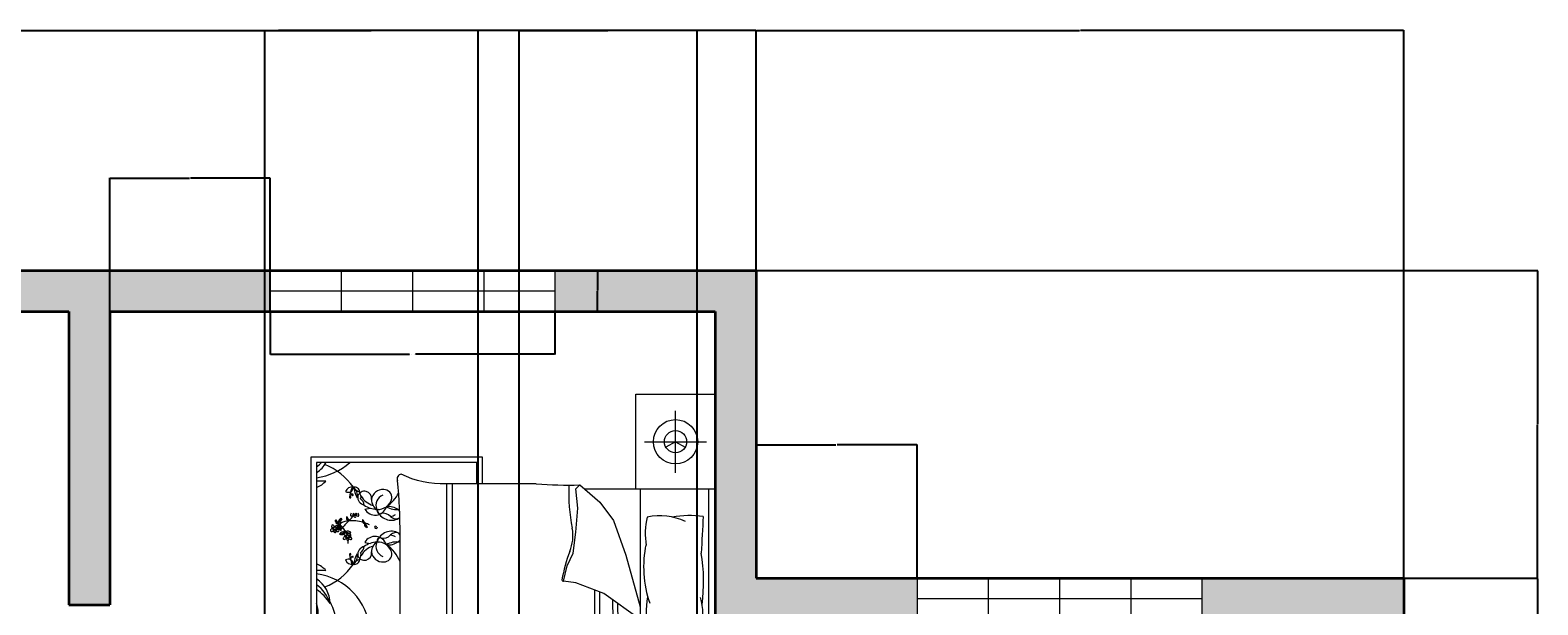
# Model space of a CAD drawing. Units: centimetres. Extents: x 2178 to 3635, y 1064 to 2635.
# Tile 9 of 9: x 2788 to 3635, y 2312 to 2635. Entities that reach past the tile are written whole.
import ezdxf

# ---------------------------------------------------------------- set-up
doc = ezdxf.new("R2010")
doc.units = ezdxf.units.CM
for name, color, linetype, lineweight in [('A-ANNO-DIMS', 2, 'Continuous', 18), ('A-FURN', 42, 'Continuous', 18), ('A-GLAZ', 4, 'Continuous', 18), ('A-WALL', 7, 'Continuous', 35)]:
    doc.layers.add(name, color=color, linetype=linetype, lineweight=lineweight)
doc.layers.add('A-WALL-PATT', color=18, linetype='Continuous', lineweight=13, true_color=0x000000)
doc.styles.get("Standard").update_dxf_attribs({"font": 'arial.ttf'})
doc.dimstyles.get("Standard").update_dxf_attribs({"dimtxt": 0.18, "dimasz": 0.18, "dimexe": 0.18, "dimexo": 0.0625, "dimgap": 0.09, "dimtad": 0, "dimtih": 1, "dimtoh": 1, "dimdec": 4, "dimzin": 0, "dimdsep": 46, "dimtxsty": 'Standard', "dimcen": 0.09, "dimadec": 0, "dimazin": 0, "dimtfac": 1, "dimtdec": 4, "dimtofl": 0, "dimtmove": 0, "dimatfit": 3, "dimfxl": 1, "dimtolj": 1, "dimtzin": 0, "dimarcsym": 0})

# ---------------------------------------------------------------- blocks, each defined once
blk = doc.blocks.new('bed')
for p, q in [((2798.77, 2937.13), (3098.77, 2937.13)), ((2858.77, 2937.13), (2858.77, 2854.79)), ((3038.77, 2933.28), (2858.77, 2933.28)), ((2828.77, 2892.53), (2828.77, 2931.73)), ((3068.77, 2892.53), (3068.77, 2931.73)), ((2848.37, 2912.13), (2809.17, 2912.13)), ((3049.17, 2912.13), (3088.37, 2912.13)), ((2858.77, 2889.72), (3038.77, 2889.72)), ((2900.44, 2880.8), (2933.16, 2889.72)), ((2941.19, 2889.72), (2924.75, 2866.84)), ((2878.57, 2872.91), (2900.44, 2880.8)), ((3037.97, 2877.26), (2931.16, 2875.76)), ((2867.02, 2864.41), (2878.57, 2872.91)), ((2924.75, 2866.84), (2918.06, 2849.23)), ((3037.85, 2874.18), (2928.92, 2872.64)), ((2856.09, 2851.66), (2867.02, 2864.41)), ((3037.71, 2861.65), (2922.6, 2861.18)), ((3037.69, 2864.73), (2923.78, 2864.28)), ((2858.52, 2849.23), (2856.09, 2851.66)), ((2870.67, 2850.44), (2858.52, 2849.23)), ((2885.86, 2849.23), (2870.67, 2850.44)), ((2899.23, 2847.41), (2885.86, 2849.23)), ((2907.13, 2843.76), (2899.23, 2847.41)), ((2918.06, 2849.23), (2916.85, 2841.33)), ((2916.85, 2841.33), (2907.13, 2843.76)), ((2838.37, 2790.07), (2855.34, 2790.07)), ((2838.37, 2682), (2838.37, 2790.07)), ((3040.44, 2790.07), (3057.08, 2790.07)), ((3057.08, 2790.07), (3057.08, 2682)), ((2855.33, 2786.59), (2841.85, 2786.59)), ((2841.85, 2786.59), (2841.85, 2685.48)), ((3053.6, 2786.59), (3040.38, 2786.59)), ((3053.6, 2685.48), (3053.6, 2786.59)), ((3040.13, 2771.36), (2855.32, 2771.36)), ((3040.42, 2767.62), (2855.31, 2767.62)), ((3009.67, 2738.15), (2887.87, 2738.15)), ((2871.41, 2715.89), (2870.75, 2719.28)), ((2892.38, 2715.89), (2893.04, 2719.28)), ((3003.07, 2715.89), (3002.41, 2719.28)), ((3024.04, 2715.89), (3024.7, 2719.28)), ((2841.85, 2685.48), (3053.6, 2685.48)), ((3057.08, 2682), (2838.37, 2682))]:
    blk.add_line(p, q)
for points in [[(2858.77, 2887.13), (2798.77, 2887.13), (2798.77, 2937.13)], [(3038.77, 2937.13), (3038.77, 2887.13), (3098.77, 2887.13), (3098.77, 2937.13)], [(2828.77, 2912.13), (2832.27, 2918.19)], [(3068.77, 2912.13), (3065.27, 2918.19)], [(2828.77, 2912.13), (2832.27, 2906.07)], [(3068.77, 2912.13), (3065.27, 2906.07)]]:
    blk.add_lwpolyline(points)
for points in [[(2876, 2929.65, 0.074897), (2876.37, 2910.06, -0.472817)], [(2947.37, 2908.96, 0.14099), (2947.97, 2928.95, 0.235245)], [(2960.18, 2908.96, -0.14099), (2959.58, 2928.95, -0.235245)], [(3021.54, 2929.65, -0.074897), (3021.18, 2910.06, 0.472817)], [(2855.46, 2824.19, 0.001242), (2855.31, 2767.26, -0.127202), (2849.3, 2738.9)], [(3040.05, 2773.72, 0.056112), (3042.23, 2757.21, 0.095341), (3046.45, 2741.32)]]:
    blk.add_lwpolyline(points, format="xyb")
for centre, radius in [((2828.77, 2912.13), 14), ((3068.77, 2912.13), 14), ((2828.77, 2912.13), 7), ((3068.77, 2912.13), 7), ((2888.74, 2705.02), 0.764), ((3006.71, 2705.02), 0.764), ((2883.74, 2696.97), 0.764), ((3011.71, 2696.97), 0.764)]:
    blk.add_circle(centre, radius)
for centre, radius, start, end in [((3041.36, 5784.66), 2859.79, 266.68521, 267.14978), ((2917.11, 2821.09), 108.8, 82.21958, 99.49698), ((2940.09, 2876.08), 53.46, 81.52493, 103.95996), ((2963.69, 2914.69), 14.84, 63.34374, 106.10256), ((2985.93, 2877.16), 52.74, 76.34271, 101.1841), ((2856.18, 5784.66), 2859.79, 272.85022, 273.31479), ((2914.22, 2902.19), 38.67, 155.1316, 191.75834), ((2983.32, 2902.19), 38.67, 348.24166, 24.8684), ((2912, 2898.93), 36.76, 354.01289, 15.82928), ((2995.54, 2898.93), 36.76, 164.17072, 185.98711), ((2907.87, 2961.74), 69.73, 258.03974, 289.26152), ((2936.1, 2946.52), 52.9, 259.86169, 283.62376), ((2965.7, 2909.52), 15.9, 245.01826, 288.54073), ((2993.49, 2930.2), 38.19, 243.87611, 286.17464), ((2886.7, 2933.16), 40.2, 255.10393, 281.03689), ((3010.84, 2933.16), 40.2, 258.96311, 284.89607), ((3576.57, 2853.06), 539.05, 176.09997, 180.92818), ((2581.02, 2844.2), 275.17, 355.82941, 1.55305), ((2888.28, 2822.94), 24.42, 66.26158, 101.3392), ((2861.22, 2957.89), 113.22, 267.45188, 281.3392), ((2937.68, 2954.7), 116.34, 250.11942, 259.33829), ((2916.17, 2841.09), 0.724, 268.86235, 19.75363), ((3740.68, 2833.46), 703.17, 179.11454, 184.87351), ((2852.06, 2739.09), 2.77, 183.97998, 297.34124), ((2884.29, 2425.86), 312.3, 89.34325, 95.68869), ((2864.12, 2727.92), 5.07, 84.48557, 181.05378), ((2850.89, 2717.02), 22.71, 33.66712, 63.29966), ((2862.56, 2724.18), 9.02, 355.29334, 76.921), ((2881.32, 2730.53), 11.57, 145.78505, 184.73037), ((2859.22, 2735.93), 12.43, 328.82178, 9.15542), ((2874.61, 2734.83), 3.61, 120.0293, 142.32497), ((2868.85, 2732.7), 9.56, 289.28218, 29.1751), ((2867.4, 2730.97), 8.62, 7.43599, 29.91487), ((2873.09, 2735.54), 4.49, 311.56531, 23.83541), ((2874.61, 2734.83), 3.61, 44.45169, 63.55801), ((2894.94, 2732.7), 9.56, 150.8249, 250.71782), ((2890.7, 2735.54), 4.49, 156.16459, 228.43469), ((2889.17, 2734.83), 3.61, 113.22901, 135.54831), ((2896.38, 2730.97), 8.62, 150.08513, 172.56401), ((2889.17, 2734.83), 3.61, 37.67503, 66.71436), ((2882.46, 2730.53), 11.57, 355.26963, 34.21495), ((2904.56, 2735.93), 12.43, 169.71335, 211.17822), ((2901.22, 2724.18), 9.02, 103.079, 184.70666), ((2912.89, 2717.02), 22.71, 111.49413, 146.33288), ((2899.66, 2727.92), 5.07, 358.94622, 95.51443), ((2995.79, 2727.92), 5.07, 84.48557, 181.05378), ((2982.56, 2717.02), 22.71, 33.66712, 68.50587), ((2994.23, 2724.18), 9.02, 355.29334, 76.921), ((3012.99, 2730.53), 11.57, 145.78505, 184.73037), ((2990.89, 2735.93), 12.43, 328.82178, 10.28665), ((3006.28, 2734.83), 3.61, 113.28564, 142.32497), ((3000.51, 2732.7), 9.56, 289.28218, 29.1751), ((2999.07, 2730.97), 8.62, 7.43599, 29.91487), ((3006.28, 2734.83), 3.61, 44.45169, 66.71436), ((3004.75, 2735.54), 4.49, 311.56531, 23.83541), ((3018.86, 2446.37), 291.92, 85.24024, 91.80351), ((3026.6, 2732.7), 9.56, 150.8249, 250.71782), ((3022.36, 2735.54), 4.49, 156.16459, 228.43469), ((3020.84, 2734.83), 3.61, 106.63434, 135.54831), ((3028.05, 2730.97), 8.62, 150.08513, 172.56401), ((3020.84, 2734.83), 3.61, 37.67503, 72.58143), ((3014.13, 2730.53), 11.57, 355.26963, 34.21495), ((3036.23, 2735.93), 12.43, 169.24899, 211.17822), ((3032.89, 2724.18), 9.02, 103.079, 184.70666), ((3044.56, 2717.02), 22.71, 113.64533, 146.33288), ((3031.33, 2727.92), 5.07, 358.94622, 95.51443), ((3044.17, 2739.79), 2.73, 246.52186, 33.82642), ((2866.2, 2727.2), 7.17, 174.94485, 262.88575), ((2869.01, 2729.92), 6.96, 201.58187, 291.42215), ((2864.95, 2728.79), 8.71, 272.3591, 324.04014), ((2855.49, 2724.42), 16.1, 326.28828, 356.5076), ((2867.69, 2722.36), 7.46, 299.90854, 73.1337), ((2881.32, 2730.53), 11.57, 212.70113, 216.34448), ((2872.41, 2725.49), 1.86, 257.30406, 15.14713), ((2880.15, 2727.58), 6.15, 131.56531, 195.14713), ((2882.69, 2723.02), 0.94, 280.43845, 100.41356), ((2883.64, 2727.58), 6.15, 344.85287, 48.43469), ((2896.09, 2722.36), 7.46, 106.8663, 240.09146), ((2891.37, 2725.49), 1.86, 164.85287, 282.69594), ((2882.46, 2730.53), 11.57, 323.65552, 327.29887), ((2898.83, 2728.79), 8.71, 215.95986, 267.6409), ((2894.77, 2729.92), 6.96, 248.57785, 338.41813), ((2908.3, 2724.42), 16.1, 183.4924, 213.71172), ((2897.59, 2727.2), 7.17, 277.11425, 5.05515), ((2997.86, 2727.2), 7.17, 174.94485, 262.88575), ((3000.68, 2729.92), 6.96, 201.58187, 291.42215), ((2996.62, 2728.79), 8.71, 272.3591, 324.04014), ((2987.15, 2724.42), 16.1, 326.28828, 356.5076), ((2999.36, 2722.36), 7.46, 299.90854, 73.1337), ((3012.99, 2730.53), 11.57, 212.70113, 216.34448), ((3004.08, 2725.49), 1.86, 257.30406, 15.14713), ((3011.81, 2727.58), 6.15, 131.56531, 195.14713), ((3012.76, 2723.02), 0.94, 79.58644, 259.56155), ((3015.3, 2727.58), 6.15, 344.85287, 48.43469), ((3027.76, 2722.36), 7.46, 106.8663, 240.09146), ((3023.04, 2725.49), 1.86, 164.85287, 282.69594), ((3014.13, 2730.53), 11.57, 323.65552, 327.29887), ((3030.5, 2728.79), 8.71, 215.95986, 267.6409), ((3026.44, 2729.92), 6.96, 248.57785, 338.41813), ((3039.96, 2724.42), 16.1, 183.4924, 213.71172), ((3029.25, 2727.2), 7.17, 277.11425, 5.05515), ((2864.55, 2715.65), 4.5, 80.26398, 250.86884), ((2855.62, 2725.56), 14.16, 301.26137, 341.7045), ((2863.47, 2717), 5.62, 265.96902, 344.3045), ((2869.52, 2709.53), 5.99, 96.1662, 141.58255), ((2879.44, 2713.73), 1.58, 101.32561, 154.46214), ((2877.17, 2719.07), 4.74, 280.25878, 300.65599), ((2878.27, 2722.86), 8.46, 268.32639, 277.13024), ((2903.55, 2707.57), 24.85, 163.58418, 183.82768), ((2876.15, 2719.06), 4.82, 308.21012, 316.30712), ((2879.11, 2715.89), 1.44, 278.34322, 4.28685), ((2878.31, 2717.16), 2.51, 300.65599, 332.63414), ((2880.2, 2715.5), 0.611, 55.76575, 157.44165), ((2903.55, 2707.57), 24.85, 153.0032, 159.89408), ((2881.15, 2716.07), 0.611, 84.37838, 186.05427), ((2880.58, 2718.52), 2.51, 269.18588, 301.16403), ((2881.32, 2717.22), 1.44, 237.53317, 323.47681), ((2879.92, 2721.32), 4.82, 285.51291, 293.60991), ((2883.07, 2715.9), 1.58, 87.35788, 140.49441), ((2879.43, 2720.42), 4.74, 301.16403, 321.56124), ((2882.75, 2722.67), 0.578, 102.70507, 280.43845), ((2875.57, 2721.25), 8.46, 324.68979, 333.49364), ((2908.16, 2725.56), 14.16, 198.2955, 238.73863), ((2894.26, 2709.53), 5.99, 38.41745, 83.8338), ((2900.32, 2717), 5.62, 195.6955, 274.03098), ((2899.24, 2715.65), 4.5, 289.13116, 99.73602), ((2951.1, 2680.2), 39.18, 94.46233, 172.25504), ((2951.27, 2716.33), 4.34, 137.78732, 219.11446), ((2946.34, 2716.47), 3.27, 298.5391, 58.36268), ((2951.26, 2719.13), 3.2, 177.75849, 283.85198), ((2951.17, 2718.35), 3.25, 63.02737, 163.80375), ((2947.89, 2725.94), 6.69, 271.45846, 315.37266), ((2950.61, 2713.61), 6.19, 45.54113, 114.31008), ((2956.25, 2745.4), 27.41, 252.59304, 267.25817), ((2957.43, 2722.47), 9.91, 198.91595, 238.01098), ((2954.84, 2713.61), 6.19, 65.68992, 134.45887), ((2949.2, 2745.4), 27.41, 272.74183, 287.40696), ((2951.92, 2716.43), 0.424, 283.85198, 219.92454), ((2952.44, 2714.47), 0.487, 238.01098, 71.55918), ((2952.52, 2714.71), 0.236, 71.55918, 188.01668), ((2953.01, 2714.47), 0.487, 108.44082, 301.98902), ((2954.28, 2718.35), 3.25, 16.19625, 116.97263), ((2957.56, 2725.94), 6.69, 224.62734, 268.54154), ((2952.93, 2714.71), 0.236, 351.98332, 108.44082), ((2953.49, 2716.59), 0.255, 320.19092, 256.02088), ((2948.02, 2722.47), 9.91, 301.98902, 341.08405), ((2954.19, 2719.13), 3.2, 256.14802, 2.24151), ((2959.11, 2716.47), 3.27, 121.63732, 241.4609), ((2954.18, 2716.33), 4.34, 320.88554, 42.21268), ((2953.08, 2689.24), 30.32, 352.86355, 81.81966), ((2996.21, 2715.65), 4.5, 80.26398, 250.86884), ((2987.29, 2725.56), 14.16, 301.26137, 341.7045), ((2995.13, 2717), 5.62, 265.96902, 344.3045), ((3001.19, 2709.53), 5.99, 96.1662, 141.58255), ((3012.38, 2715.9), 1.58, 39.50559, 92.64212), ((3016.02, 2720.42), 4.74, 218.43876, 238.83597), ((3019.88, 2721.25), 8.46, 206.50636, 215.31021), ((3012.7, 2722.67), 0.578, 259.56155, 77.29493), ((3014.13, 2717.22), 1.44, 216.52319, 302.46683), ((3014.87, 2718.52), 2.51, 238.83597, 270.81412), ((3015.53, 2721.32), 4.82, 246.39009, 254.48709), ((2991.9, 2707.57), 24.85, 20.10592, 26.9968), ((3014.3, 2716.07), 0.611, 353.94573, 95.62162), ((3016.34, 2715.89), 1.44, 175.71315, 261.65678), ((3015.25, 2715.5), 0.611, 22.55835, 124.23425), ((3017.14, 2717.16), 2.51, 207.36586, 239.34401), ((2991.9, 2707.57), 24.85, 356.17232, 16.41582), ((3019.3, 2719.06), 4.82, 223.69288, 231.78988), ((3018.28, 2719.07), 4.74, 239.34401, 259.74122), ((3017.18, 2722.86), 8.46, 262.86976, 271.67361), ((3016.01, 2713.73), 1.58, 25.53786, 78.67439), ((3039.83, 2725.56), 14.16, 198.2955, 238.73863), ((3031.98, 2717), 5.62, 195.6955, 274.03098), ((3025.93, 2709.53), 5.99, 38.41745, 83.8338), ((3030.9, 2715.65), 4.5, 289.13116, 99.73602), ((2812.68, 2680.2), 39.18, 7.74496, 41.8856), ((2879.7, 2676.32), 39.18, 124.38655, 158.59079), ((2860.73, 2709.42), 3.25, 92.95159, 193.72796), ((2861.82, 2707.73), 4.34, 167.71153, 249.03868), ((2854.09, 2714.37), 6.69, 301.38267, 345.29688), ((2862.6, 2705.03), 6.19, 75.46535, 144.23429), ((2851.64, 2735.41), 27.41, 282.51726, 297.18239), ((2857.48, 2705.38), 3.27, 328.46331, 88.28689), ((2864.1, 2716.11), 9.91, 228.84017, 267.9352), ((2860.42, 2710.14), 3.2, 207.6827, 313.77619), ((2863.62, 2710.77), 2.76, 63.97555, 143.26805), ((2862.34, 2708.13), 0.424, 313.77619, 249.71835), ((2863.71, 2706.94), 0.236, 101.4834, 217.94089), ((2863.76, 2706.7), 0.487, 267.9352, 101.4834), ((2874.99, 2710.74), 1.27, 101.56373, 142.6358), ((2873.93, 2709.56), 0.764, 273.27684, 86.72316), ((2874.97, 2708.15), 1.26, 217.76209, 259.04026), ((2874.82, 2710.28), 0.73, 91.10805, 181.86747), ((2876.33, 2709.83), 2.32, 203.42757, 227.61037), ((2875.59, 2708.82), 1.58, 80.3487, 133.65382), ((2875.31, 2710.12), 1.25, 229.78892, 317.67915), ((2873.96, 2711.74), 1.84, 288.72627, 352.50315), ((2873.9, 2707.47), 1.78, 355.05304, 68.36176), ((2875.3, 2707.17), 2.5, 83.08516, 105.71709), ((2875.21, 2711.65), 0.59, 345.23556, 144.9248), ((2875.09, 2707.37), 0.586, 232.47371, 355.05304), ((2857.98, 2686.43), 28.48, 43.15413, 52.0459), ((2875.75, 2709.72), 0.658, 317.67915, 80.3487), ((2877.65, 2703.63), 1.58, 101.32561, 154.46214), ((2875.39, 2708.98), 4.74, 280.25878, 300.65599), ((2876.48, 2712.77), 8.46, 268.32639, 277.13024), ((2874.36, 2708.97), 4.82, 308.21012, 316.30712), ((2877.32, 2705.8), 1.44, 278.34322, 4.28685), ((2876.52, 2707.06), 2.51, 300.65599, 332.63414), ((2878.41, 2705.4), 0.611, 55.76575, 157.44165), ((2891.17, 2706.94), 12.46, 184.75602, 209.20408), ((2909.1, 2733.46), 40.99, 222.24124, 232.17444), ((2884.75, 2705.38), 2.12, 272.84988, 356.12261), ((2882.89, 2706.16), 3.48, 304.53686, 16.36991), ((2883.26, 2704.56), 2.05, 321.76073, 7.92519), ((2887.73, 2705.18), 2.46, 127.31045, 187.92519), ((2884.34, 2705.45), 2.53, 355.01064, 41.65801), ((2888.54, 2702.71), 2.41, 104.75581, 148.0499), ((2887.9, 2706.08), 1.04, 126.10456, 271.42811), ((2887.78, 2706.37), 0.749, 353.75256, 131.70535), ((2887.61, 2704.38), 0.506, 262.90601, 7.13198), ((2887.08, 2705.48), 1.05, 0.06451, 61.15075), ((2887.33, 2706.37), 1.2, 311.84125, 355.78771), ((2889.8, 2706.2), 1.27, 101.56373, 176.36503), ((2889.63, 2705.74), 0.73, 91.10805, 181.86747), ((2891.14, 2705.29), 2.32, 203.42757, 227.61037), ((2890.41, 2704.28), 1.58, 80.3487, 133.65382), ((2890.12, 2705.58), 1.25, 229.78892, 317.67915), ((2888.77, 2707.2), 1.84, 288.72627, 352.50315), ((2888.71, 2702.93), 1.78, 355.05304, 68.36176), ((2890.11, 2702.63), 2.5, 83.08516, 105.71709), ((2890.02, 2707.11), 0.59, 345.23556, 144.9248), ((2890.56, 2705.18), 0.658, 317.67915, 80.3487), ((2892.45, 2690.4), 14.94, 87.10709, 94.75853), ((2900.16, 2710.77), 2.76, 36.73195, 116.02445), ((2900.02, 2706.7), 0.487, 78.5166, 272.0648), ((2901.18, 2705.03), 6.19, 35.76571, 104.53465), ((2912.15, 2735.41), 27.41, 242.81761, 257.48274), ((2899.68, 2716.11), 9.91, 272.0648, 311.15983), ((2900.07, 2706.94), 0.236, 322.05911, 78.5166), ((2903.37, 2710.14), 3.2, 226.22381, 332.3173), ((2901.49, 2708.3), 0.255, 290.26671, 226.22708), ((2906.3, 2705.38), 3.27, 91.71311, 211.53669), ((2903.05, 2709.42), 3.25, 346.27204, 87.04841), ((2909.69, 2714.37), 6.69, 194.70312, 238.61733), ((2901.96, 2707.73), 4.34, 290.96132, 12.28847), ((2884.08, 2676.32), 39.18, 21.40921, 55.61345), ((3011.37, 2676.32), 39.18, 124.38655, 158.59079), ((2993.49, 2707.73), 4.34, 167.71153, 249.03868), ((2992.4, 2709.42), 3.25, 92.95159, 193.72796), ((2985.76, 2714.37), 6.69, 301.38267, 345.29688), ((2994.27, 2705.03), 6.19, 75.46535, 144.23429), ((2983.3, 2735.41), 27.41, 282.51726, 297.18239), ((2992.08, 2710.14), 3.2, 207.6827, 313.77619), ((2995.76, 2716.11), 9.91, 228.84017, 267.9352), ((2989.15, 2705.38), 3.27, 328.46331, 88.28689), ((2995.29, 2710.77), 2.76, 63.97555, 143.26805), ((2994.01, 2708.13), 0.424, 313.77619, 249.71835), ((2995.38, 2706.94), 0.236, 101.4834, 217.94089), ((2995.43, 2706.7), 0.487, 267.9352, 101.4834), ((3003, 2690.4), 14.94, 85.24147, 92.89291), ((3004.89, 2705.18), 0.658, 99.6513, 222.32085), ((3005.33, 2705.58), 1.25, 222.32085, 310.21108), ((3005.04, 2704.28), 1.58, 46.34618, 99.6513), ((3005.43, 2707.11), 0.59, 35.0752, 194.76444), ((3006.68, 2707.2), 1.84, 187.49685, 251.27373), ((3006.74, 2702.93), 1.78, 111.63824, 184.94696), ((3005.34, 2702.63), 2.5, 74.28291, 96.91484), ((3005.82, 2705.74), 0.73, 358.13253, 88.89195), ((3004.31, 2705.29), 2.32, 312.38963, 336.57243), ((3005.65, 2706.2), 1.27, 3.63497, 78.43627), ((3007.67, 2706.37), 0.749, 48.29465, 186.24744), ((3008.12, 2706.37), 1.2, 184.21229, 228.15875), ((3008.37, 2705.48), 1.05, 118.84925, 179.93549), ((3007.84, 2704.38), 0.506, 172.86802, 277.09399), ((3007.55, 2706.08), 1.04, 268.57189, 53.89544), ((3006.91, 2702.71), 2.41, 31.9501, 75.24419), ((3011.11, 2705.45), 2.53, 138.34199, 184.98936), ((3010.7, 2705.38), 2.12, 183.87739, 267.15012), ((3012.56, 2706.16), 3.48, 163.63009, 235.46314), ((3007.72, 2705.18), 2.46, 352.07481, 52.68955), ((3012.19, 2704.56), 2.05, 172.07481, 218.23927), ((2986.35, 2733.46), 40.99, 307.82556, 317.75876), ((3004.28, 2706.94), 12.46, 330.79592, 355.24398), ((3037.47, 2686.43), 28.48, 127.9541, 136.84587), ((3017.04, 2705.4), 0.611, 22.55835, 124.23425), ((3018.13, 2705.8), 1.44, 175.71315, 261.65678), ((3018.93, 2707.06), 2.51, 207.36586, 239.34401), ((3021.09, 2708.97), 4.82, 223.69288, 231.78988), ((3020.06, 2708.98), 4.74, 239.34401, 259.74122), ((3018.97, 2712.77), 8.46, 262.86976, 271.67361), ((3017.8, 2703.63), 1.58, 25.53786, 78.67439), ((3019.7, 2709.72), 0.658, 99.6513, 222.32085), ((3020.14, 2710.12), 1.25, 222.32085, 310.21108), ((3019.86, 2708.82), 1.58, 46.34618, 99.6513), ((3020.24, 2711.65), 0.59, 35.0752, 194.76444), ((3021.49, 2711.74), 1.84, 187.49685, 251.27373), ((3021.55, 2707.47), 1.78, 111.63824, 184.94696), ((3020.36, 2707.37), 0.586, 184.94696, 307.52629), ((3020.15, 2707.17), 2.5, 74.28291, 96.91484), ((3020.63, 2710.28), 0.73, 358.13253, 88.89195), ((3019.12, 2709.83), 2.32, 312.38963, 336.57243), ((3020.46, 2710.74), 1.27, 37.3642, 78.43627), ((3020.48, 2708.15), 1.26, 280.95974, 322.23791), ((3021.52, 2709.56), 0.764, 93.27684, 266.72316), ((3031.83, 2710.77), 2.76, 36.73195, 116.02445), ((3031.69, 2706.7), 0.487, 78.5166, 272.0648), ((3032.85, 2705.03), 6.19, 35.76571, 104.53465), ((3043.81, 2735.41), 27.41, 242.81761, 257.48274), ((3031.35, 2716.11), 9.91, 272.0648, 311.15983), ((3031.74, 2706.94), 0.236, 322.05911, 78.5166), ((3035.03, 2710.14), 3.2, 226.22381, 332.3173), ((3033.16, 2708.3), 0.255, 290.26671, 226.22708), ((3037.97, 2705.38), 3.27, 91.71311, 211.53669), ((3041.36, 2714.37), 6.69, 194.70312, 238.61733), ((3034.72, 2709.42), 3.25, 346.27204, 87.04841), ((3033.63, 2707.73), 4.34, 290.96132, 12.28847), ((3015.75, 2676.32), 39.18, 21.40921, 55.61345), ((3082.77, 2680.2), 39.18, 138.1144, 172.25504), ((2878.18, 2700.87), 0.853, 146.86359, 236.90213), ((2890.21, 2719.66), 22.32, 235.1882, 238.88441), ((2879.65, 2702.11), 2.31, 199.47987, 267.68284), ((2879.39, 2701.23), 1.99, 212.81548, 277.39917), ((2878.23, 2699.91), 2.31, 266.97007, 338.29129), ((2866.06, 2716.39), 22.32, 302.6784, 306.37461), ((2878.82, 2698.08), 0.853, 214.3538, 304.39233), ((2879.13, 2701.31), 0.883, 238.88441, 314.26458), ((2878.94, 2699.33), 1.99, 280.30568, 17.1958), ((2878.77, 2699.13), 0.883, 306.37461, 21.75478), ((2880.21, 2699.7), 0.666, 19.36054, 201.75478), ((2880.22, 2700.2), 0.666, 311.87034, 134.26458), ((2892.74, 2694.13), 13.31, 153.78194, 158.29129), ((2882.15, 2703.22), 3.48, 247.23048, 319.06353), ((2881, 2702.05), 2.05, 264.45436, 310.61881), ((2891.17, 2706.94), 12.46, 214.00334, 222.49171), ((2882.5, 2701.23), 2.12, 218.32082, 298.81623), ((2892.45, 2690.4), 14.94, 120.54402, 139.81798), ((2882.14, 2695.53), 0.757, 148.0499, 225.62681), ((2883.54, 2694.66), 2.41, 104.75581, 148.0499), ((2882.19, 2696.38), 1.51, 247.40857, 351.43859), ((2882.9, 2698.03), 1.04, 126.10456, 271.42811), ((2882.78, 2698.31), 0.749, 353.75256, 131.70535), ((2883.94, 2698.62), 2.46, 70.00407, 130.61881), ((2882.61, 2696.32), 0.506, 262.90601, 7.13198), ((2882.08, 2697.42), 1.05, 0.06451, 61.15075), ((2882.33, 2698.32), 1.2, 311.84125, 355.78771), ((2882.35, 2701.62), 2.53, 297.70426, 344.35163), ((2884.78, 2695.55), 1.26, 151.21959, 259.04026), ((2884.8, 2698.15), 1.27, 101.56373, 176.36503), ((2884.63, 2697.69), 0.73, 91.10805, 181.86747), ((2886.15, 2697.23), 2.32, 203.42757, 227.61037), ((2885.41, 2696.22), 1.58, 80.3487, 133.65382), ((2885.13, 2697.53), 1.25, 229.78892, 317.67915), ((2883.78, 2699.15), 1.84, 288.72627, 352.50315), ((2883.72, 2694.88), 1.78, 355.05304, 68.36176), ((2885.11, 2694.58), 2.5, 83.08516, 105.71709), ((2885.03, 2699.06), 0.59, 345.23556, 144.9248), ((2883.69, 2701.61), 2.05, 8.72271, 54.88717), ((2883.8, 2699.97), 3.48, 0.278, 72.11105), ((2885.36, 2701.25), 2.12, 20.5253, 88.5375), ((2885.56, 2697.13), 0.658, 317.67915, 80.3487), ((2888.15, 2702.29), 2.46, 188.72271, 249.33746), ((2887.13, 2703.59), 0.757, 148.0499, 225.62681), ((2892.45, 2690.4), 14.94, 113.05007, 113.84774), ((2887.18, 2704.44), 1.51, 247.40857, 351.43859), ((2884.99, 2701.06), 2.53, 334.9899, 21.63727), ((2889.78, 2703.61), 1.26, 151.21959, 259.04026), ((2889.9, 2702.83), 0.586, 232.47371, 355.05304), ((2948.1, 2659.21), 39.18, 94.46233, 117.4146), ((2948.27, 2695.35), 4.34, 137.78732, 219.11446), ((2943.34, 2695.48), 3.27, 298.5391, 58.36268), ((2948.26, 2698.14), 3.2, 177.75849, 283.85198), ((2948.18, 2697.36), 3.25, 63.02737, 163.80375), ((2944.89, 2704.96), 6.69, 271.45846, 315.37266), ((2947.61, 2692.63), 6.19, 45.54113, 114.31008), ((2954.43, 2701.48), 9.91, 198.91595, 238.01098), ((2953.26, 2724.42), 27.41, 252.59304, 267.25817), ((2948.92, 2695.44), 0.424, 283.85198, 219.92454), ((2957.84, 2692.63), 6.19, 65.68992, 134.45887), ((2952.19, 2724.42), 27.41, 272.74183, 287.40696), ((2957.27, 2697.36), 3.25, 16.19625, 116.97263), ((2960.56, 2704.96), 6.69, 224.62734, 268.54154), ((2956.49, 2695.61), 0.255, 320.19092, 256.02088), ((2951.02, 2701.48), 9.91, 301.98902, 341.08405), ((2957.19, 2698.14), 3.2, 256.14802, 2.24151), ((2962.11, 2695.48), 3.27, 121.63732, 241.4609), ((2957.18, 2695.35), 4.34, 320.88554, 42.21268), ((2957.35, 2659.21), 39.18, 62.5854, 85.53767), ((3005.55, 2702.83), 0.586, 184.94696, 307.52629), ((3005.67, 2703.61), 1.26, 280.95974, 28.78041), ((3008.27, 2704.44), 1.51, 188.56141, 292.59143), ((3010.46, 2701.06), 2.53, 158.36273, 205.0101), ((3010.09, 2701.25), 2.12, 91.4625, 159.4747), ((3011.65, 2699.97), 3.48, 107.88895, 179.722), ((3007.3, 2702.29), 2.46, 290.66254, 351.27729), ((3008.32, 2703.59), 0.757, 314.37319, 31.9501), ((3003, 2690.4), 14.94, 66.15226, 66.94993), ((3009.89, 2697.13), 0.658, 99.6513, 222.32085), ((3010.32, 2697.53), 1.25, 222.32085, 310.21108), ((3011.76, 2701.61), 2.05, 125.11283, 171.27729), ((3010.04, 2696.22), 1.58, 46.34618, 99.6513), ((3010.42, 2699.06), 0.59, 35.0752, 194.76444), ((3011.67, 2699.15), 1.84, 187.49685, 251.27373), ((3011.73, 2694.88), 1.78, 111.63824, 184.94696), ((3010.34, 2694.58), 2.5, 74.28291, 96.91484), ((3003, 2690.4), 14.94, 40.18202, 59.45598), ((3011.51, 2698.62), 2.46, 49.38119, 109.99593), ((3013.3, 2703.22), 3.48, 220.93647, 292.76952), ((3013.1, 2701.62), 2.53, 195.64837, 242.29574), ((3010.82, 2697.69), 0.73, 358.13253, 88.89195), ((3009.3, 2697.23), 2.32, 312.38963, 336.57243), ((3010.65, 2698.15), 1.27, 3.63497, 78.43627), ((3010.67, 2695.55), 1.26, 280.95974, 28.78041), ((3013.26, 2696.38), 1.51, 188.56141, 292.59143), ((3012.67, 2698.31), 0.749, 48.29465, 186.24744), ((3013.12, 2698.32), 1.2, 184.21229, 228.15875), ((3012.95, 2701.23), 2.12, 241.18377, 321.67918), ((3013.37, 2697.42), 1.05, 118.84925, 179.93549), ((3012.84, 2696.32), 0.506, 172.86802, 277.09399), ((3012.55, 2698.03), 1.04, 268.57189, 53.89544), ((3011.91, 2694.66), 2.41, 31.9501, 75.24419), ((3014.45, 2702.05), 2.05, 229.38119, 275.54564), ((3004.28, 2706.94), 12.46, 317.50829, 325.99666), ((3013.31, 2695.53), 0.757, 314.37319, 31.9501), ((3016.51, 2699.33), 1.99, 162.8042, 259.69432), ((3015.23, 2700.2), 0.666, 45.73542, 228.12966), ((3015.24, 2699.7), 0.666, 338.24522, 160.63946), ((3002.71, 2694.13), 13.31, 21.70871, 26.21806), ((3017.22, 2699.91), 2.31, 201.70871, 273.02993), ((3016.32, 2701.31), 0.883, 225.73542, 301.11559), ((3016.68, 2699.13), 0.883, 158.24522, 233.62539), ((3016.06, 2701.23), 1.99, 262.60083, 327.18452), ((3015.8, 2702.11), 2.31, 272.31716, 340.52013), ((3029.39, 2716.39), 22.32, 233.62539, 237.3216), ((3016.63, 2698.08), 0.853, 235.60767, 325.6462), ((3005.24, 2719.66), 22.32, 301.11559, 304.8118), ((3017.27, 2700.87), 0.853, 303.09787, 33.13641), ((2832.33, 2674.95), 19.09, 33.46172, 60.11157), ((2825.46, 2671.39), 23.79, 36.30357, 46.48142), ((2843.02, 2679.37), 15.93, 22.55474, 48.95456), ((2799.39, 2687.93), 54.2, 357.40811, 3.65191), ((2884.9, 2694.78), 0.586, 232.47371, 355.05304), ((2920.76, 2679.37), 15.93, 131.04544, 157.44526), ((2964.39, 2687.93), 54.2, 176.34809, 182.59189), ((2931.45, 2674.95), 19.09, 91.27197, 146.53828), ((2938.32, 2671.39), 23.79, 107.85038, 143.69643), ((2950.82, 2664.7), 35.39, 124.01234, 144.05304), ((2937.15, 2664.88), 21.54, 73.54311, 107.0202), ((2945.68, 2653.78), 31.85, 94.37872, 95.63574), ((2962.46, 2631.95), 56.92, 109.72171, 109.90284), ((2949.44, 2693.49), 0.487, 238.01098, 71.55918), ((2949.52, 2693.73), 0.236, 71.55918, 188.01668), ((2956.01, 2693.49), 0.487, 108.44082, 301.98902), ((2955.93, 2693.73), 0.236, 351.98332, 108.44082), ((2968.3, 2664.88), 21.54, 72.9798, 106.45689), ((2959.77, 2653.78), 31.85, 84.36426, 85.62128), ((2942.99, 2631.95), 56.92, 70.09716, 70.27829), ((2957, 2692.01), 17.54, 338.11703, 6.61954), ((2973.09, 2687.13), 7.03, 346.38982, 79.07385), ((2967.81, 2688.1), 8.89, 342.86088, 41.90487), ((2931.06, 2687.93), 54.2, 357.40811, 3.65191), ((2974.69, 2679.37), 15.93, 22.55474, 48.95456), ((3010.55, 2694.78), 0.586, 184.94696, 307.52629), ((3052.43, 2679.37), 15.93, 131.04544, 157.44526), ((3096.06, 2687.93), 54.2, 176.34809, 182.59189), ((3063.12, 2674.95), 19.09, 119.88843, 146.53828), ((3069.99, 2671.39), 23.79, 133.51858, 143.69643)]:
    blk.add_arc(centre, radius, start, end)
blk = doc.blocks.new('WIN-1600-4LT')
for p, q in [((0, 23), (0, 0)), ((40, 23), (40, 0)), ((80, 23), (80, 0)), ((120, 23), (120, 0)), ((160, 23), (160, 0)), ((0, 11.5), (160, 11.5))]:
    blk.add_line(p, q)
blk = doc.blocks.new('*D24')
at = {"layer": 'A-ANNO-DIMS', "color": 0, "lineweight": -2, "transparency": 16777216}
for p, q in [((2922.6, 2476.53), (2922.6, 2452.41)), ((3082.6, 2476.53), (3082.6, 2452.41)), ((2922.78, 2452.59), (3000.9, 2452.59)), ((3082.42, 2452.59), (3004.31, 2452.59))]:
    blk.add_line(p, q, dxfattribs=at)
at = {"layer": 'A-ANNO-DIMS', "color": 0, "transparency": 16777216}
for points in [[(2922.78, 2452.62), (2922.78, 2452.56), (2922.6, 2452.59)], [(3082.42, 2452.62), (3082.42, 2452.56), (3082.6, 2452.59)]]:
    blk.add_solid(points, dxfattribs=at)
at = {"layer": 'Defpoints', "color": 0, "transparency": 16777216}
for p in [(2922.6, 2476.59), (3082.6, 2476.59), (3082.6, 2452.59)]:
    blk.add_point(p, dxfattribs=at)
at = {"layer": 'A-ANNO-DIMS', "color": 0, "transparency": 16777216, "insert": (3002.6, 2452.59), "char_height": 0.18, "attachment_point": 5}
blk.add_mtext('\\A1;4-LIGHT WINDOW 160 TYP.', dxfattribs=at)
blk = doc.blocks.new('*D25')
at = {"layer": 'A-ANNO-DIMS', "color": 0, "lineweight": -2, "transparency": 16777216}
for p, q in [((3082.67, 2499.59), (3106.78, 2499.59)), ((3106.6, 2499.41), (3106.6, 2488.27)), ((3106.6, 2476.77), (3106.6, 2487.91)), ((3082.67, 2476.59), (3106.78, 2476.59))]:
    blk.add_line(p, q, dxfattribs=at)
at = {"layer": 'A-ANNO-DIMS', "color": 0, "transparency": 16777216}
for points in [[(3106.57, 2499.41), (3106.63, 2499.41), (3106.6, 2499.59)], [(3106.57, 2476.77), (3106.63, 2476.77), (3106.6, 2476.59)]]:
    blk.add_solid(points, dxfattribs=at)
at = {"layer": 'Defpoints', "color": 0, "transparency": 16777216}
for p in [(3082.6, 2499.59), (3106.6, 2499.59), (3082.6, 2476.59)]:
    blk.add_point(p, dxfattribs=at)
at = {"layer": 'A-ANNO-DIMS', "color": 0, "transparency": 16777216, "insert": (3106.6, 2488.09), "char_height": 0.18, "attachment_point": 5}
blk.add_mtext('\\A1;23 TYP.', dxfattribs=at)
blk = doc.blocks.new('*D50')
at = {"layer": 'A-ANNO-DIMS', "color": 0, "lineweight": -2, "transparency": 16777216}
for p, q in [((2658.56, 2559.65), (2658.56, 2634.77)), ((2658.74, 2634.59), (2926.79, 2634.59)), ((3195.42, 2634.59), (2927.37, 2634.59)), ((3195.6, 2499.65), (3195.6, 2634.77))]:
    blk.add_line(p, q, dxfattribs=at)
at = {"layer": 'A-ANNO-DIMS', "color": 0, "transparency": 16777216}
for points in [[(2658.74, 2634.62), (2658.74, 2634.56), (2658.56, 2634.59)], [(3195.42, 2634.62), (3195.42, 2634.56), (3195.6, 2634.59)]]:
    blk.add_solid(points, dxfattribs=at)
at = {"layer": 'Defpoints', "color": 0, "transparency": 16777216}
for p in [(3195.6, 2634.59), (2658.56, 2559.59), (3195.6, 2499.59)]:
    blk.add_point(p, dxfattribs=at)
at = {"layer": 'A-ANNO-DIMS', "color": 0, "transparency": 16777216, "insert": (2927.08, 2634.59), "char_height": 0.18, "attachment_point": 5}
blk.add_mtext('\\A1;537', dxfattribs=at)
blk = doc.blocks.new('*D51')
at = {"layer": 'A-ANNO-DIMS', "color": 0, "lineweight": -2, "transparency": 16777216}
for p, q in [((3195.6, 2499.65), (3195.6, 2634.77)), ((3195.78, 2634.59), (3377.32, 2634.59)), ((3559.42, 2634.59), (3377.89, 2634.59)), ((3559.6, 2326.65), (3559.6, 2634.77))]:
    blk.add_line(p, q, dxfattribs=at)
at = {"layer": 'A-ANNO-DIMS', "color": 0, "transparency": 16777216}
for points in [[(3195.78, 2634.62), (3195.78, 2634.56), (3195.6, 2634.59)], [(3559.42, 2634.62), (3559.42, 2634.56), (3559.6, 2634.59)]]:
    blk.add_solid(points, dxfattribs=at)
at = {"layer": 'Defpoints', "color": 0, "transparency": 16777216}
for p in [(3559.6, 2634.59), (3195.6, 2499.59), (3559.6, 2326.59)]:
    blk.add_point(p, dxfattribs=at)
at = {"layer": 'A-ANNO-DIMS', "color": 0, "transparency": 16777216, "insert": (3377.6, 2634.59), "char_height": 0.18, "attachment_point": 5}
blk.add_mtext('\\A1;364', dxfattribs=at)
blk = doc.blocks.new('*D53')
at = {"layer": 'A-ANNO-DIMS', "color": 0, "lineweight": -2, "transparency": 16777216}
for p, q in [((3195.67, 2499.59), (3634.78, 2499.59)), ((3634.6, 2499.41), (3634.6, 2413.27)), ((3634.6, 2326.77), (3634.6, 2412.91)), ((3195.67, 2326.59), (3634.78, 2326.59))]:
    blk.add_line(p, q, dxfattribs=at)
at = {"layer": 'A-ANNO-DIMS', "color": 0, "transparency": 16777216}
for points in [[(3634.57, 2499.41), (3634.63, 2499.41), (3634.6, 2499.59)], [(3634.57, 2326.77), (3634.63, 2326.77), (3634.6, 2326.59)]]:
    blk.add_solid(points, dxfattribs=at)
at = {"layer": 'Defpoints', "color": 0, "transparency": 16777216}
for p in [(3195.6, 2499.59), (3634.6, 2499.59), (3195.6, 2326.59)]:
    blk.add_point(p, dxfattribs=at)
at = {"layer": 'A-ANNO-DIMS', "color": 0, "transparency": 16777216, "insert": (3634.6, 2413.09), "char_height": 0.18, "attachment_point": 5}
blk.add_mtext('\\A1;173', dxfattribs=at)
blk = doc.blocks.new('*D54')
at = {"layer": 'A-ANNO-DIMS', "color": 0, "lineweight": -2, "transparency": 16777216}
for p, q in [((3559.67, 2326.59), (3634.78, 2326.59)), ((3634.6, 2326.41), (3634.6, 2283.77)), ((3634.6, 2240.77), (3634.6, 2283.41)), ((3559.67, 2240.59), (3634.78, 2240.59))]:
    blk.add_line(p, q, dxfattribs=at)
at = {"layer": 'A-ANNO-DIMS', "color": 0, "transparency": 16777216}
for points in [[(3634.57, 2326.41), (3634.63, 2326.41), (3634.6, 2326.59)], [(3634.57, 2240.77), (3634.63, 2240.77), (3634.6, 2240.59)]]:
    blk.add_solid(points, dxfattribs=at)
at = {"layer": 'Defpoints', "color": 0, "transparency": 16777216}
for p in [(3559.6, 2326.59), (3634.6, 2326.59), (3559.6, 2240.59)]:
    blk.add_point(p, dxfattribs=at)
at = {"layer": 'A-ANNO-DIMS', "color": 0, "transparency": 16777216, "insert": (3634.6, 2283.59), "char_height": 0.18, "attachment_point": 5}
blk.add_mtext('\\A1;86', dxfattribs=at)
blk = doc.blocks.new('*D61')
at = {"layer": 'A-ANNO-DIMS', "color": 0, "lineweight": -2, "transparency": 16777216}
for p, q in [((2919.6, 1623.65), (2919.6, 2634.77)), ((2919.78, 2634.59), (2979.32, 2634.59)), ((3039.42, 2634.59), (2979.88, 2634.59)), ((3039.6, 1623.65), (3039.6, 2634.77))]:
    blk.add_line(p, q, dxfattribs=at)
at = {"layer": 'A-ANNO-DIMS', "color": 0, "transparency": 16777216}
for points in [[(2919.78, 2634.62), (2919.78, 2634.56), (2919.6, 2634.59)], [(3039.42, 2634.62), (3039.42, 2634.56), (3039.6, 2634.59)]]:
    blk.add_solid(points, dxfattribs=at)
at = {"layer": 'Defpoints', "color": 0, "transparency": 16777216}
for p in [(3039.6, 2634.59), (2919.6, 1623.59), (3039.6, 1623.59)]:
    blk.add_point(p, dxfattribs=at)
at = {"layer": 'A-ANNO-DIMS', "color": 0, "transparency": 16777216, "insert": (2979.6, 2634.59), "char_height": 0.18, "attachment_point": 5}
blk.add_mtext('\\A1;120', dxfattribs=at)
blk = doc.blocks.new('*D62')
at = {"layer": 'A-ANNO-DIMS', "color": 0, "lineweight": -2, "transparency": 16777216}
for p, q in [((3062.6, 1623.65), (3062.6, 2634.77)), ((3062.78, 2634.59), (3112.32, 2634.59)), ((3162.42, 2634.59), (3112.88, 2634.59)), ((3162.6, 1623.65), (3162.6, 2634.77))]:
    blk.add_line(p, q, dxfattribs=at)
at = {"layer": 'A-ANNO-DIMS', "color": 0, "transparency": 16777216}
for points in [[(3062.78, 2634.62), (3062.78, 2634.56), (3062.6, 2634.59)], [(3162.42, 2634.62), (3162.42, 2634.56), (3162.6, 2634.59)]]:
    blk.add_solid(points, dxfattribs=at)
at = {"layer": 'Defpoints', "color": 0, "transparency": 16777216}
for p in [(3162.6, 2634.59), (3062.6, 1623.59), (3162.6, 1623.59)]:
    blk.add_point(p, dxfattribs=at)
at = {"layer": 'A-ANNO-DIMS', "color": 0, "transparency": 16777216, "insert": (3112.6, 2634.59), "char_height": 0.18, "attachment_point": 5}
blk.add_mtext('\\A1;100', dxfattribs=at)
blk = doc.blocks.new('*D76')
at = {"layer": 'A-ANNO-DIMS', "color": 0, "lineweight": -2, "transparency": 16777216}
for p, q in [((2832.6, 2476.65), (2832.6, 2551.77)), ((2832.78, 2551.59), (2877.39, 2551.59)), ((2922.42, 2551.59), (2877.82, 2551.59)), ((2922.6, 2476.65), (2922.6, 2551.77))]:
    blk.add_line(p, q, dxfattribs=at)
at = {"layer": 'A-ANNO-DIMS', "color": 0, "transparency": 16777216}
for points in [[(2832.78, 2551.62), (2832.78, 2551.56), (2832.6, 2551.59)], [(2922.42, 2551.62), (2922.42, 2551.56), (2922.6, 2551.59)]]:
    blk.add_solid(points, dxfattribs=at)
at = {"layer": 'Defpoints', "color": 0, "transparency": 16777216}
for p in [(2922.6, 2551.59), (2832.6, 2476.59), (2922.6, 2476.59)]:
    blk.add_point(p, dxfattribs=at)
at = {"layer": 'A-ANNO-DIMS', "color": 0, "transparency": 16777216, "insert": (2877.6, 2551.59), "char_height": 0.18, "attachment_point": 5}
blk.add_mtext('\\A1;90', dxfattribs=at)
blk = doc.blocks.new('*D77')
at = {"layer": 'A-ANNO-DIMS', "color": 0, "lineweight": -2, "transparency": 16777216}
for p, q in [((3195.6, 2326.65), (3195.6, 2401.77)), ((3195.78, 2401.59), (3240.53, 2401.59)), ((3285.92, 2401.59), (3241.18, 2401.59)), ((3286.1, 2326.65), (3286.1, 2401.77))]:
    blk.add_line(p, q, dxfattribs=at)
at = {"layer": 'A-ANNO-DIMS', "color": 0, "transparency": 16777216}
for points in [[(3195.78, 2401.62), (3195.78, 2401.56), (3195.6, 2401.59)], [(3285.92, 2401.62), (3285.92, 2401.56), (3286.1, 2401.59)]]:
    blk.add_solid(points, dxfattribs=at)
at = {"layer": 'Defpoints', "color": 0, "transparency": 16777216}
for p in [(3286.1, 2401.59), (3195.6, 2326.59), (3286.1, 2326.59)]:
    blk.add_point(p, dxfattribs=at)
at = {"layer": 'A-ANNO-DIMS', "color": 0, "transparency": 16777216, "insert": (3240.85, 2401.59), "char_height": 0.18, "attachment_point": 5}
blk.add_mtext('\\A1;90.5', dxfattribs=at)

msp = doc.modelspace()

# ---------------------------------------------------------------- hatches: boundary and pattern name
at = {"layer": 'A-WALL-PATT'}
h = msp.add_hatch(color=256, dxfattribs=at)
h.dxf.hatch_style = 1
h.paths.add_polyline_path([(2276.605, 2499.59), (2253.605, 2499.59), (2253.605, 2476.59), (2276.605, 2476.59)])
h.paths.add_polyline_path([(2411.605, 2350.59), (2253.605, 2350.59), (2253.605, 2327.59), (2411.605, 2327.59)])
h.paths.add_polyline_path([(2276.605, 2252.59), (2253.605, 2252.59), (2253.605, 2020.59), (2276.605, 2020.59), (2276.605, 2093.59), (2561.605, 2093.59), (2561.605, 2116.59), (2276.605, 2116.59)])
h.paths.add_polyline_path([(2659.605, 1787.59), (2610.616, 1787.59), (2276.605, 1787.59), (2276.605, 1860.59), (2253.605, 1860.59), (2253.605, 1732.09), (2276.605, 1732.09), (2276.605, 1764.59), (2516.605, 1764.59), (2516.605, 1699.59), (2539.605, 1699.59), (2539.605, 1764.59), (2659.605, 1764.59)])
h.paths.add_polyline_path([(2539.605, 1624.59), (2276.605, 1624.59), (2276.605, 1657.09), (2253.605, 1657.09), (2253.605, 1561.59), (2276.605, 1561.59), (2276.605, 1601.59), (2539.605, 1601.59)])
h.paths.add_polyline_path([(2276.605, 1501.59), (2253.605, 1501.59), (2253.605, 1371.59), (2276.605, 1371.59)])
h.paths.add_polyline_path([(2376.605, 1271.59), (2276.605, 1271.59), (2276.605, 1311.59), (2253.605, 1311.59), (2253.605, 1248.59), (2376.605, 1248.59)])
h.paths.add_polyline_path([(2636.605, 1271.59), (2536.605, 1271.59), (2536.605, 1248.59), (2636.605, 1248.59)])
h.paths.add_polyline_path([(2659.605, 1600.59), (2919.605, 1600.59), (2919.605, 1623.59), (2636.605, 1623.59), (2636.605, 1188.59), (2659.605, 1188.59)])
h.paths.add_polyline_path([(2939.605, 1211.59), (2759.605, 1211.59), (2759.605, 1188.59), (2939.605, 1188.59)])
h.paths.add_polyline_path([(3062.605, 1288.59), (3039.605, 1288.59), (3039.605, 1188.59), (3062.605, 1188.59)])
h.paths.add_polyline_path([(3372.605, 1248.59), (3062.605, 1248.59), (3062.605, 1218.59), (3372.605, 1218.59)])
h.paths.add_polyline_path([(3395.605, 1271.59), (3372.605, 1271.59), (3372.605, 1248.59), (3395.605, 1248.59)])
h.paths.add_polyline_path([(3559.605, 1271.59), (3536.605, 1271.59), (3536.605, 1248.59), (3559.605, 1248.59)])
h.paths.add_polyline_path([(3559.605, 1623.59), (3536.605, 1623.59), (3536.605, 1600.59), (3559.605, 1600.59)])
h.paths.add_polyline_path([(3395.605, 1623.59), (3162.605, 1623.59), (3162.605, 1600.59), (3395.605, 1600.59)])
h.paths.add_polyline_path([(3395.605, 1411.59), (3277.1, 1411.59), (3277.1, 1388.59), (3395.605, 1388.59)])
h.paths.add_polyline_path([(3157.1, 1411.59), (3062.605, 1411.59), (3062.605, 1623.59), (3039.605, 1623.59), (3039.605, 1388.59), (3157.1, 1388.59)])
h.paths.add_polyline_path([(3559.605, 1797.09), (3536.605, 1797.09), (3536.605, 1764.59), (3316.605, 1764.59), (3316.605, 1927.59), (3293.605, 1927.59), (3293.605, 1741.59), (3372.605, 1741.59), (3395.605, 1741.59), (3559.605, 1741.59)])
h.paths.add_polyline_path([(3559.605, 1990.59), (3536.605, 1990.59), (3536.605, 1974.446), (3536.605, 1927.59), (3391.605, 1927.59), (3391.605, 1904.59), (3536.605, 1904.59), (3536.605, 1872.09), (3559.605, 1872.09)])
h.paths.add_polyline_path([(3559.605, 2180.59), (3536.605, 2180.59), (3536.605, 2050.59), (3559.605, 2050.59)])
h.paths.add_polyline_path([(3559.605, 2326.59), (3446.105, 2326.59), (3446.105, 2303.59), (3536.605, 2303.59), (3536.605, 2240.59), (3559.605, 2240.59)])
h.paths.add_polyline_path([(3286.105, 2326.59), (3195.605, 2326.59), (3195.605, 2499.59), (3082.605, 2499.59), (3082.605, 2476.59), (3172.605, 2476.59), (3172.605, 2116.59), (2809.605, 2116.59), (2809.605, 2093.59), (3172.605, 2093.59), (3172.605, 1904.59), (3195.605, 1904.59), (3195.605, 2303.59), (3286.105, 2303.59)])
h.paths.add_polyline_path([(2832.605, 2236.59), (2659.605, 2236.59), (2659.605, 2476.59), (2697.105, 2476.59), (2697.105, 2499.59), (2636.605, 2499.59), (2636.605, 2093.59), (2699.605, 2093.59), (2699.605, 2116.59), (2659.605, 2116.59), (2659.605, 2213.59), (2832.605, 2213.59)])
h.paths.add_polyline_path([(2832.605, 2476.59), (2922.605, 2476.59), (2922.605, 2499.59), (2772.105, 2499.59), (2772.105, 2476.59), (2809.605, 2476.59), (2809.605, 2311.59), (2832.605, 2311.59)])

# ---------------------------------------------------------------- linework, layer by layer
at = {"layer": 'A-WALL'}
for p, q in [((2636.605, 2499.59), (3195.605, 2499.59)), ((3195.605, 2499.59), (3195.605, 2326.59)), ((2659.605, 2476.59), (2809.605, 2476.59)), ((2809.605, 2476.59), (2809.605, 2311.59)), ((2832.605, 2476.59), (2832.605, 2311.59)), ((2832.605, 2476.59), (3172.605, 2476.59)), ((3172.605, 2476.59), (3172.605, 2116.59)), ((3195.605, 2326.59), (3559.605, 2326.59)), ((3559.605, 2326.59), (3559.605, 1188.59)), ((2809.605, 2311.59), (2832.605, 2311.59))]:
    msp.add_line(p, q, dxfattribs=at)

# ---------------------------------------------------------------- block references
at = {"layer": 'A-FURN', "xscale": 0.8894661318613604, "yscale": 0.8894661318613604, "zscale": 0.8894661318613604, "rotation": 270}
msp.add_blockref('bed', (560.128, 4919.422), dxfattribs=at)
at = {"layer": 'A-GLAZ'}
for p in [(2922.605, 2476.59), (3286.105, 2303.59)]:
    msp.add_blockref('WIN-1600-4LT', p, dxfattribs=at)

# ---------------------------------------------------------------- dimensions: what is measured, and where the dimension line sits
at = {"layer": 'A-ANNO-DIMS'}
for base, p1, p2, override, picture, middle in [((3195.605, 2634.59), (2658.563, 2559.59), (3195.605, 2499.59), {"dimdec": 0, "dimlfac": 1, "dimrnd": 0, "dimzin": 0, "dimdsep": 46, "dimlunit": 2}, '*D50', (2927.084, 2634.59)), ((3039.605, 2634.59), (2919.605, 1623.59), (3039.605, 1623.59), {"dimdec": 0, "dimlfac": 1, "dimrnd": 0, "dimzin": 0, "dimdsep": 46, "dimlunit": 2}, '*D61', (2979.605, 2634.59)), ((3162.605, 2634.59), (3062.605, 1623.59), (3162.605, 1623.59), {"dimdec": 0, "dimlfac": 1, "dimrnd": 0, "dimzin": 0, "dimdsep": 46, "dimlunit": 2}, '*D62', (3112.605, 2634.59)), ((3559.605, 2634.59), (3195.605, 2499.59), (3559.605, 2326.59), {"dimdec": 0, "dimlfac": 1, "dimrnd": 0, "dimzin": 0, "dimdsep": 46, "dimlunit": 2}, '*D51', (3377.605, 2634.59)), ((2922.605, 2551.59), (2832.605, 2476.59), (2922.605, 2476.59), {"dimdec": 0, "dimlfac": 1, "dimrnd": 0, "dimzin": 0, "dimdsep": 46, "dimlunit": 2}, '*D76', (2877.605, 2551.59)), ((3286.105, 2401.59), (3195.605, 2326.59), (3286.105, 2326.59), {"dimdec": 1, "dimlfac": 1, "dimrnd": 0, "dimzin": 0, "dimdsep": 46, "dimlunit": 2}, '*D77', (3240.855, 2401.59))]:
    dim = msp.add_linear_dim(base=base, p1=p1, p2=p2, dimstyle='Standard', override=override, dxfattribs=at)
    dim.commit()
    dim.dimension.update_dxf_attribs({"geometry": picture, "text_midpoint": middle})
dim = msp.add_linear_dim(base=(3106.605, 2499.59), p1=(3082.605, 2476.59), p2=(3082.605, 2499.59), angle=90, text='<> TYP.', dimstyle='Standard', override={"dimdec": 0, "dimlfac": 1, "dimrnd": 0, "dimzin": 0, "dimdsep": 46, "dimlunit": 2}, dxfattribs=at)
dim.commit()
dim.dimension.update_dxf_attribs({"geometry": '*D25', "text_midpoint": (3106.605, 2488.09)})
for base, p1, p2, picture, middle in [((3634.605, 2499.59), (3195.605, 2326.59), (3195.605, 2499.59), '*D53', (3634.605, 2413.09)), ((3634.605, 2326.59), (3559.605, 2240.59), (3559.605, 2326.59), '*D54', (3634.605, 2283.59))]:
    dim = msp.add_linear_dim(base=base, p1=p1, p2=p2, angle=90, dimstyle='Standard', override={"dimdec": 0, "dimlfac": 1, "dimrnd": 0, "dimzin": 0, "dimdsep": 46, "dimlunit": 2}, dxfattribs=at)
    dim.commit()
    dim.dimension.update_dxf_attribs({"geometry": picture, "text_midpoint": middle})
dim = msp.add_linear_dim(base=(3082.605, 2452.59), p1=(2922.605, 2476.59), p2=(3082.605, 2476.59), text='4-LIGHT WINDOW <> TYP.', dimstyle='Standard', override={"dimdec": 0, "dimlfac": 1, "dimrnd": 0, "dimzin": 0, "dimdsep": 46, "dimlunit": 2}, dxfattribs=at)
dim.commit()
dim.dimension.update_dxf_attribs({"geometry": '*D24', "text_midpoint": (3002.605, 2452.59)})

doc.saveas('drawing.dxf')
